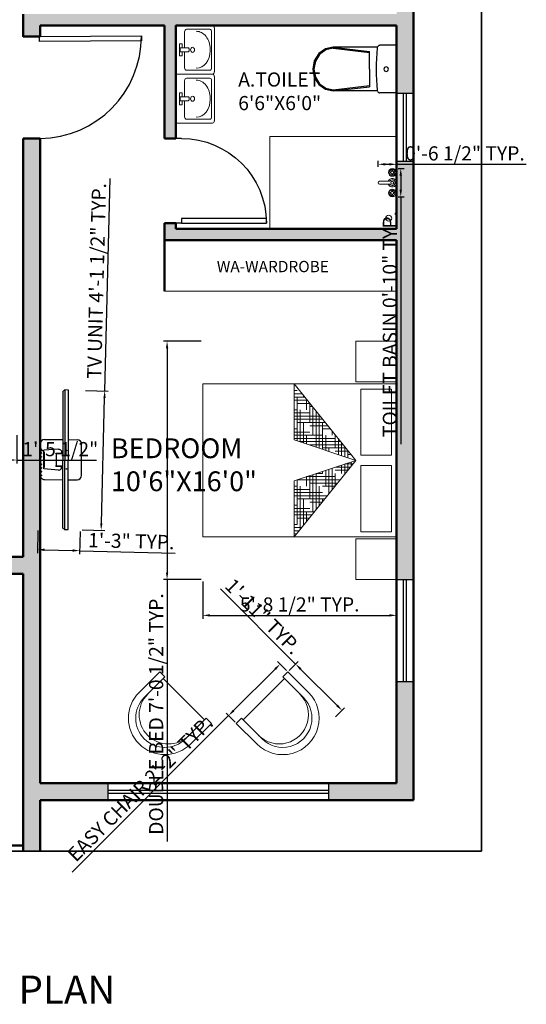
# Model space of a CAD drawing. Units: inches. Extents: x 2638 to 4577, y 1946 to 2619.
# Tile 5 of 8: x 3284 to 3463, y 1946 to 2294. Entities that reach past the tile are written whole.
import ezdxf

# ---------------------------------------------------------------- set-up
doc = ezdxf.new("R2010")
doc.units = ezdxf.units.IN
for name, color, linetype, lineweight in [('A-ANNO-DIMS', 2, 'Continuous', 18), ('A-ANNO-TEXT', 7, 'Continuous', 25), ('A-AREA-IDEN', 7, 'Continuous', 25), ('A-DOOR', 4, 'Continuous', 25), ('A-FLOR-FIXT', 8, 'Continuous', 18), ('A-FURN', 8, 'Continuous', 18), ('A-GLAZ', 4, 'Continuous', 25), ('A-WALL', 7, 'Continuous', 50), ('A-WALL-PATT', 8, 'Continuous', 13), ('C-PROP', 1, 'Continuous', 35)]:
    doc.layers.add(name, color=color, linetype=linetype, lineweight=lineweight)
doc.layers.add('SANTEH', color=7, linetype='Continuous')
doc.layers.add('window', color=130, linetype='Continuous')
doc.styles.get("Standard").update_dxf_attribs({"font": 'arial.ttf'})
doc.dimstyles.new('ISO-25', dxfattribs={"dimtxt": 5, "dimasz": 2.5, "dimexe": 1.25, "dimexo": 0.625, "dimtad": 1, "dimdec": 1, "dimlunit": 3, "dimtxsty": 'Standard', "dimcen": 2.5, "dimclrt": 1, "dimadec": 0, "dimazin": 0, "dimtfac": 1, "dimtdec": 1, "dimtmove": 0, "dimatfit": 3, "dimfxl": 1, "dimarcsym": 0})

# ---------------------------------------------------------------- blocks, each defined once
blk = doc.blocks.new('*U5')
for p, q in [((0, 0), (0, -6)), ((30, 0), (30, -6))]:
    blk.add_line(p, q)
blk.add_lwpolyline([(0, 0), (0, 30), (1.75, 30), (1.75, 0)], close=True)
blk.add_arc((0, 0), 30, 0, 90)
blk = doc.blocks.new('*U4')
for p, q in [((0, 0), (0, -6)), ((36, 0), (36, -6))]:
    blk.add_line(p, q)
blk.add_lwpolyline([(0, 0), (0, 36), (1.75, 36), (1.75, 0)], close=True)
blk.add_arc((0, 0), 36, 0, 90)
blk = doc.blocks.new('TV')
at = {"color": 0}
for p, q in [((3967.27, 1784.85), (3967.05, 1784.65)), ((3967.76, 1763.68), (3967.54, 1763.86))]:
    blk.add_line(p, q, dxfattribs=at)
at = {"layer": 'window'}
for p, q in [((3967.54, 1763.86), (3967.05, 1784.65)), ((3964.41, 1777.23), (3967.22, 1777.3)), ((3968.01, 1777.32), (3969.36, 1777.35)), ((3966.53, 1775.82), (3964.33, 1775.61)), ((3964.34, 1775.34), (3964.45, 1775.34)), ((3964.34, 1775.31), (3964.43, 1775.32)), ((3966.14, 1775.2), (3967.01, 1775.22)), ((3966.14, 1775.18), (3967.27, 1775.2)), ((3966.14, 1775.18), (3966.14, 1775.2)), ((3966.3, 1773.29), (3966.26, 1775.18)), ((3964.39, 1773.06), (3964.48, 1773.06)), ((3964.39, 1773.04), (3964.5, 1773.04)), ((3966.19, 1773.28), (3967.31, 1773.31)), ((3966.19, 1773.26), (3967.05, 1773.28)), ((3966.19, 1773.26), (3966.19, 1773.28)), ((3966.61, 1772.66), (3964.4, 1772.77)), ((3964.55, 1771.15), (3967.36, 1771.22)), ((3968.15, 1771.24), (3969.5, 1771.27))]:
    blk.add_line(p, q, dxfattribs=at)
for points in [[(3968.33, 1763.69), (3967.83, 1784.86), (3967.27, 1784.85), (3967.76, 1763.68), (3968.33, 1763.69)], [(3963.86, 1771.81), (3963.75, 1776.54)], [(3970.16, 1771.96), (3970.05, 1776.69)], [(3964.4, 1772.77), (3964.33, 1775.61)], [(3964.48, 1773.06), (3964.43, 1775.32)], [(3964.5, 1773.04), (3964.45, 1775.34)]]:
    blk.add_lwpolyline(points, dxfattribs=at)
for points in [[(3966.53, 1775.82, -0.263666), (3966.93, 1775.69), (3967, 1775.57), (3967.01, 1775.22)], [(3966.61, 1772.66, 0.263666), (3967, 1772.81), (3967.06, 1772.93), (3967.05, 1773.28)]]:
    blk.add_lwpolyline(points, format="xyb", dxfattribs=at)
for centre, radius in [((3963.91, 1775.73), 0.0679), ((3963.93, 1775.17), 0.0679), ((3963.94, 1774.6), 0.0679), ((3967.77, 1775.68), 0.0451), ((3963.95, 1774.04), 0.0679), ((3963.97, 1773.48), 0.0679), ((3963.98, 1772.92), 0.0679), ((3967.83, 1772.86), 0.0451), ((3963.99, 1772.35), 0.0679), ((3964.01, 1771.79), 0.0679)]:
    blk.add_circle(centre, radius, dxfattribs=at)
for centre, start, end in [((3964.42, 1776.56), 91.3414, 181.3414), ((3969.38, 1776.67), 1.3414, 91.3414), ((3964.53, 1771.83), 181.3414, 271.3414), ((3969.49, 1771.94), 271.3414, 1.3414)]:
    blk.add_arc(centre, 0.676, start, end, dxfattribs=at)
blk = doc.blocks.new('Rac7')
at = {"color": 0}
for p, q in [((-39501, -24232), (-39501, -23830)), ((-39474, -23808), (-38988, -23808)), ((-39457, -23859), (-39457, -24115)), ((-39032, -23838), (-39430, -23838)), ((-39221, -23855), (-39241, -23855)), ((-39005, -24115), (-39005, -23859)), ((-39005, -23859), (-39005, -23859)), ((-38961, -23830), (-38961, -24232)), ((-39253, -24186), (-39253, -24094)), ((-39209, -24186), (-39209, -24094)), ((-39430, -24136), (-39253, -24136)), ((-39297, -24164), (-39253, -24164)), ((-39297, -24194), (-39297, -24164)), ((-39165, -24194), (-39297, -24194)), ((-39253, -24186), (-39209, -24186)), ((-39209, -24136), (-39032, -24136)), ((-39209, -24164), (-39165, -24164)), ((-39165, -24164), (-39165, -24194)), ((-38961, -24232), (-39501, -24232))]:
    blk.add_line(p, q, dxfattribs=at)
at = {"color": 0, "extrusion": (0, 0, -1)}
for centre, major_axis, start_param, end_param in [((-39474, -23830), (-27, 0), 0, 1.570796), ((-39430, -23859), (-27, 0), 0, 1.570796), ((-39241, -24007), (-194, 0), 0, 1.570796), ((-39221, -24007), (-194, 0), 1.570796, 3.141593), ((-39032, -23859), (-27, 0), 1.570796, 3.141593), ((-38988, -23830), (-27, 0), 1.570796, 3.141593), ((-39231, -24104), (-25.3, 0), 0.552816, 2.588777), ((-39430, -24115), (-27, 0), -1.570796, 0), ((-39032, -24115), (-27, 0), -3.141593, -1.570796)]:
    blk.add_ellipse(centre, major_axis=major_axis, ratio=0.785714, start_param=start_param, end_param=end_param, dxfattribs=at)
blk.add_ellipse((-39231, -24048), major_axis=(-27.9, 0), ratio=0.785714, dxfattribs=at)
blk = doc.blocks.new('WC 2 Symb_109')
at = {"layer": 'SANTEH'}
for p, q in [((0, 0), (0, 380)), ((0, 380), (132.4, 380)), ((153.6, 364.9), (506.8, 364.9)), ((506.3, 364.9), (215.7, 330.9)), ((506.3, 356), (215.7, 322)), ((215.7, 190), (215.7, 330.9)), ((215.7, 190), (215.7, 49.1)), ((153.8, 15.1), (506.8, 15.1)), ((506.3, 24), (215.7, 58)), ((506.3, 15.1), (215.7, 49.1)), ((0, 0), (132.4, 0))]:
    blk.add_line(p, q, dxfattribs=at)
for points in [[(154.6, 360.1), (153.9, 364.1), (152.3, 367.9), (150.2, 371.3), (147.4, 374.3), (144.1, 376.7), (140.5, 378.5), (136.5, 379.6), (132.4, 380)], [(154.6, 19.7), (158.6, 62.1), (161.4, 104.7), (163.1, 147.3), (163.7, 189.9), (163.1, 232.5), (161.4, 275.1), (158.6, 317.7), (154.6, 360.1)], [(506.3, 24), (565.5, 36.6), (615.7, 72.6), (649.2, 126.5), (661, 190), (649.2, 253.5), (615.7, 307.4), (565.5, 343.4), (506.3, 356)], [(506.8, 15.1), (569.2, 28.4), (622.2, 66.3), (657.6, 123.1), (670, 190), (657.6, 256.9), (622.2, 313.7), (569.2, 351.6), (506.8, 364.9)], [(132.4, 0), (136.5, 0.4), (140.4, 1.5), (144.1, 3.2), (147.3, 5.6), (150.1, 8.6), (152.3, 12), (153.8, 15.7), (154.6, 19.7)]]:
    blk.add_lwpolyline(points, dxfattribs=at)
blk.add_lwpolyline([(83.6, 208.5), (70.4, 203.1), (64.9, 190), (70.4, 176.9), (83.6, 171.5), (96.8, 176.9), (102.2, 190), (96.8, 203.1)], close=True, dxfattribs=at)
blk = doc.blocks.new('Faucet - Bathroom top')
for p, q in [((-4.107, 0.125), (-4.375, 0.125)), ((-3.75, 0.4788), (-3.75, 0.75)), ((-3.5, 0.482), (-3.5, 0.75)), ((-3.1461, 0.125), (-2.875, 0.125)), ((3.143, 0.125), (2.875, 0.125)), ((3.5, 0.4788), (3.5, 0.75)), ((3.75, 0.482), (3.75, 0.75)), ((4.1039, 0.125), (4.375, 0.125)), ((-4.1039, -0.125), (-4.375, -0.125)), ((-3.75, -0.4821), (-3.75, -0.75)), ((-3.5, -0.4789), (-3.5, -0.75)), ((-3.143, -0.125), (-2.875, -0.125)), ((-0.5, -0.8639), (-0.5, -4.5)), ((0.5, -4.5), (0.5, -0.8631)), ((3.1461, -0.125), (2.875, -0.125)), ((3.5, -0.4821), (3.5, -0.75)), ((3.75, -0.4789), (3.75, -0.75)), ((4.107, -0.125), (4.375, -0.125))]:
    blk.add_line(p, q)
for centre, radius in [((-3.625, 0), 1.375), ((-4.625, 0), 0.2795), ((-3.625, 0), 0.5), ((-3.625, 1), 0.2795), ((-2.625, 0), 0.2795), ((0, 0), 0.5), ((3.625, 0), 1.375), ((2.625, 0), 0.2795), ((3.625, 0), 0.5), ((3.625, 1), 0.2795), ((4.625, 0), 0.2795), ((-3.625, -1), 0.2795), ((3.625, -1), 0.2795)]:
    blk.add_circle(centre, radius)
for centre, radius, start, end in [((-3.625, 0), 1, 105.2407, 164.2093), ((-3.625, 0), 1, 16.44125, 74.07887), ((0, 0), 1.5, 289.6514, 250.3603), ((0, 0), 1, 300.3431, 239.7554), ((3.625, 0), 1, 106.12, 164.0884), ((3.625, 0), 1, 16.23422, 73.90469), ((-3.625, 0), 1, 196.2342, 253.9047), ((-3.625, 0), 1, 286.12, 344.0884), ((3.625, 0), 1, 196.4413, 254.0789), ((3.625, 0), 1, 285.2407, 344.2093), ((0, -4.5), 0.5, 180, 0)]:
    blk.add_arc(centre, radius, start, end)
blk = doc.blocks.new('*X22')
at = {"color": 0}
for p, q in [((20.25, 14.8125), (20.2772, 14.8125)), ((20.1236, 14.6875), (20.25, 14.6875)), ((20.125, 14.5), (20.125, 14.6893)), ((20.1487, 14.7188), (20.2772, 14.7188)), ((20.1562, 14.625), (20.1562, 14.7281)), ((20.1739, 14.75), (20.2772, 14.75)), ((20.1875, 14.75), (20.1875, 14.7669)), ((20.199, 14.7812), (20.2772, 14.7812)), ((20.25, 14.3194), (20.25, 14.75)), ((20.0625, 14.2573), (20.0625, 14.6116)), ((20.0938, 14.375), (20.0938, 14.6504)), ((20.0984, 14.6562), (20.125, 14.6562)), ((20.125, 14.5938), (20.2772, 14.5938)), ((20.2188, 14.3091), (20.2188, 14.625)), ((20.25, 14.625), (20.2772, 14.625)), ((19.9727, 14.5), (20.25, 14.5)), ((19.9979, 14.5312), (20.2772, 14.5312)), ((20, 14.2366), (20, 14.5)), ((20.023, 14.5625), (20.2772, 14.5625)), ((20.0312, 14.2469), (20.0312, 14.5727)), ((20.1875, 14.2987), (20.1875, 14.5)), ((19.9062, 14.375), (19.9062, 14.4174)), ((19.9225, 14.4375), (20, 14.4375)), ((19.9476, 14.4688), (20.125, 14.4688)), ((20.125, 14.4062), (20.2772, 14.4062)), ((20.25, 14.4375), (20.2772, 14.4375)), ((19.8125, 14.1744), (19.8125, 14.3008)), ((19.8219, 14.3125), (20.2291, 14.3125)), ((19.8438, 14.1848), (19.8438, 14.3397)), ((19.875, 14.25), (19.875, 14.3785)), ((19.875, 14.3438), (20.2772, 14.3438)), ((19.9688, 14.2262), (19.9688, 14.375)), ((20, 14.375), (20.2772, 14.375)), ((20.1562, 14.2884), (20.1562, 14.375)), ((19.7465, 14.2188), (19.875, 14.2188)), ((19.75, 14.1537), (19.75, 14.2231)), ((19.7716, 14.25), (20, 14.25)), ((19.7812, 14.1641), (19.7812, 14.262)), ((19.7967, 14.2812), (20.125, 14.2812)), ((19.9375, 14.2159), (19.9375, 14.25)), ((19.7188, 14.0726), (19.7188, 14.1136)), ((19.7213, 14.1875), (19.75, 14.1875)), ((19.7018, 14.0938), (19.7786, 14.0938)), ((19.7269, 14.0625), (19.8728, 14.0625)), ((19.75, 14.0338), (19.75, 14.1032)), ((19.752, 14.0312), (19.875, 14.0312)), ((19.7812, 13.9949), (19.7812, 14.0929)), ((19.8125, 14), (19.8125, 14.0825)), ((19.9062, 13.8396), (19.9062, 14.0514)), ((19.9375, 13.8007), (19.9375, 14.0411)), ((19.9688, 13.875), (19.9688, 14.0307)), ((20, 14), (20, 14.0204)), ((19.8275, 13.9375), (20.25, 13.9375)), ((19.875, 13.8784), (19.875, 14)), ((19.875, 13.9688), (20.1557, 13.9688)), ((20, 14), (20.0614, 14)), ((20.0625, 13.6454), (20.0625, 13.9996)), ((20.0938, 13.625), (20.0938, 13.9893)), ((20.125, 13.75), (20.125, 13.9789)), ((20.1562, 13.875), (20.1562, 13.9686)), ((20.25, 13.5), (20.25, 13.9375)), ((19.8526, 13.9062), (20.125, 13.9062)), ((19.8777, 13.875), (20, 13.875)), ((20.0312, 13.6842), (20.0312, 13.875)), ((20.125, 13.8438), (20.2772, 13.8438)), ((20.2188, 13.4511), (20.2188, 13.875)), ((20.25, 13.875), (20.2772, 13.875)), ((19.9532, 13.7812), (20.2772, 13.7812)), ((19.9783, 13.75), (20.25, 13.75)), ((20, 13.8125), (20.2772, 13.8125)), ((20, 13.723), (20, 13.75)), ((20.1875, 13.49), (20.1875, 13.75)), ((20.0035, 13.7188), (20.125, 13.7188)), ((20.0789, 13.625), (20.2772, 13.625)), ((20.125, 13.6562), (20.2772, 13.6562)), ((20.1562, 13.5288), (20.1562, 13.625)), ((20.25, 13.6875), (20.2772, 13.6875)), ((20.104, 13.5938), (20.2772, 13.5938)), ((20.1292, 13.5625), (20.25, 13.5625)), ((20.2046, 13.4688), (20.2772, 13.4688)), ((20.2297, 13.4375), (20.2772, 13.4375)), ((20.25, 13.5), (20.2772, 13.5)), ((20.2549, 13.4062), (20.2772, 13.4062))]:
    blk.add_line(p, q, dxfattribs=at)
blk = doc.blocks.new('MAT-P02')
for p, q in [((-1.17, 0), (-1.17, -0.4)), ((-1.17, 0), (-0.77, 0)), ((-0.77, 0), (-0.77, -0.4)), ((-0.75, 0), (0.75, 0)), ((-0.75, 0), (-0.75, -1.9)), ((0.75, 0), (0.75, -1.9)), ((0.77, 0), (1.17, 0)), ((0.77, 0), (0.77, -0.4)), ((1.17, 0), (1.17, -0.4)), ((-0.7, -0.05), (-0.7, -0.35)), ((-0.7, -0.05), (-0.05, -0.05)), ((-0.05, -0.35), (-0.05, -0.05)), ((0.05, -0.05), (0.7, -0.05)), ((0.05, -0.35), (0.05, -0.05)), ((0.7, -0.05), (0.7, -0.35)), ((-0.7, -0.35), (-0.05, -0.35)), ((0.05, -0.35), (0.7, -0.35)), ((-1.17, -0.4), (-0.77, -0.4)), ((-0.75, -1.0034), (0, -0.4)), ((0, -0.4), (-0.75, -1.0034)), ((0, -0.4), (-0.2, -1.0034)), ((0, -0.4), (0.2, -1.0034)), ((0, -0.4), (0.75, -1.0034)), ((0.77, -0.4), (1.17, -0.4)), ((-0.75, -1.0034), (-0.2, -1.0034)), ((0.2, -1.0034), (0.75, -1.0034)), ((0.75, -1.9), (-0.75, -1.9))]:
    blk.add_line(p, q)
at = {"xscale": -1, "rotation": 90}
blk.add_blockref('*X22', (14.1285, 19.2738), dxfattribs=at)
blk = doc.blocks.new('12PSTG07')
at = {"color": 0, "linetype": 'ByBlock'}
for p, q in [((0, 15), (-12, 15)), ((0, 12), (0, 15)), ((-12, 12), (0, 12)), ((-1, -12), (-1, 12)), ((-12, -12), (0, -12)), ((0, -12), (0, -15)), ((0, -15), (-12, -15))]:
    blk.add_line(p, q, dxfattribs=at)
for centre, radius in [((-12, 0), 15), ((-12, 0), 12), ((-10, 0), 12)]:
    blk.add_arc(centre, radius, 90, 270, dxfattribs=at)
blk = doc.blocks.new('WIN-36')
for p, q in [((2761.41, 2540.16), (2761.41, 2534.16)), ((2797.41, 2540.16), (2797.41, 2534.16)), ((2761.41, 2537.66), (2797.41, 2537.66)), ((2761.41, 2536.66), (2797.41, 2536.66))]:
    blk.add_line(p, q)
blk = doc.blocks.new('WIN-24')
for p, q in [((2905.41, 2558.16), (2905.41, 2552.16)), ((2929.41, 2558.16), (2929.41, 2552.16)), ((2905.41, 2555.66), (2929.41, 2555.66)), ((2905.41, 2554.66), (2929.41, 2554.66))]:
    blk.add_line(p, q)
blk = doc.blocks.new('WIN-78')
for p, q in [((3314.99, 2024.16), (3314.99, 2018.16)), ((3392.99, 2024.16), (3392.99, 2018.16)), ((3314.99, 2021.66), (3392.99, 2021.66)), ((3314.99, 2020.66), (3392.99, 2020.66))]:
    blk.add_line(p, q)
blk = doc.blocks.new('*D59')
at = {"layer": 'A-ANNO-DIMS', "color": 0, "lineweight": -2, "transparency": 16777216}
for p, q in [((3378.15, 2064), (3374.97, 2067.18)), ((3374.09, 2064.53), (3359.39, 2049.82)), ((3357.62, 2048.05), (3302.31, 1992.75)), ((3359.91, 2045.76), (3356.74, 2048.94))]:
    blk.add_line(p, q, dxfattribs=at)
at = {"layer": 'A-ANNO-DIMS', "color": 0, "transparency": 16777216}
for points in [[(3373.8, 2064.82), (3374.39, 2064.23), (3375.86, 2066.29)], [(3359.09, 2050.12), (3359.68, 2049.53), (3357.62, 2048.05)]]:
    blk.add_solid(points, dxfattribs=at)
at = {"layer": 'Defpoints', "color": 0, "transparency": 16777216}
for p in [(3378.59, 2063.56), (3357.62, 2048.05), (3360.36, 2045.32)]:
    blk.add_point(p, dxfattribs=at)
at = {"layer": 'A-ANNO-DIMS', "color": 1, "transparency": 16777216, "insert": (3326.81, 2021.79), "char_height": 5, "attachment_point": 5, "rotation": 45}
blk.add_mtext('EASY CHAIR 2\'-2" TYP.', dxfattribs=at)
blk = doc.blocks.new('*D60')
at = {"layer": 'A-ANNO-DIMS', "color": 0, "lineweight": -2, "transparency": 16777216}
for p, q in [((3381.33, 2066.29), (3354.71, 2092.91)), ((3379.04, 2064), (3382.21, 2067.18)), ((3395.98, 2051.65), (3383.1, 2064.53)), ((3395.45, 2047.58), (3398.63, 2050.76))]:
    blk.add_line(p, q, dxfattribs=at)
at = {"layer": 'A-ANNO-DIMS', "color": 0, "transparency": 16777216}
for points in [[(3383.39, 2064.82), (3382.8, 2064.23), (3381.33, 2066.29)], [(3396.27, 2051.94), (3395.68, 2051.35), (3397.75, 2049.88)]]:
    blk.add_solid(points, dxfattribs=at)
at = {"layer": 'Defpoints', "color": 0, "transparency": 16777216}
for p in [(3381.33, 2066.29), (3378.59, 2063.56), (3395.01, 2047.14)]:
    blk.add_point(p, dxfattribs=at)
at = {"layer": 'A-ANNO-DIMS', "color": 1, "transparency": 16777216, "insert": (3369.36, 2082.7), "char_height": 5, "attachment_point": 5, "rotation": 315}
blk.add_mtext('1\'-11" TYP.', dxfattribs=at)
blk = doc.blocks.new('*D67')
at = {"layer": 'A-ANNO-DIMS', "color": 0, "lineweight": -2, "transparency": 16777216}
for p, q in [((3313.83, 2162.87), (3315.74, 2237.96)), ((3307.06, 2163.05), (3315.08, 2162.84)), ((3312.64, 2116.09), (3313.76, 2160.38)), ((3305.8, 2113.76), (3313.82, 2113.56))]:
    blk.add_line(p, q, dxfattribs=at)
at = {"layer": 'A-ANNO-DIMS', "color": 0, "transparency": 16777216}
for points in [[(3313.35, 2160.39), (3314.18, 2160.37), (3313.83, 2162.87)], [(3312.22, 2116.1), (3313.05, 2116.08), (3312.57, 2113.59)]]:
    blk.add_solid(points, dxfattribs=at)
at = {"layer": 'Defpoints', "color": 0, "transparency": 16777216}
for p in [(3306.43, 2163.06), (3313.83, 2162.87), (3305.18, 2113.78)]:
    blk.add_point(p, dxfattribs=at)
at = {"layer": 'A-ANNO-DIMS', "color": 1, "transparency": 16777216, "insert": (3311.6, 2201.75), "char_height": 5, "attachment_point": 5, "rotation": 88.5431}
blk.add_mtext('TV UNIT 4\'-1 1/2" TYP.', dxfattribs=at)
blk = doc.blocks.new('*D68')
at = {"layer": 'A-ANNO-DIMS', "color": 0, "lineweight": -2, "transparency": 16777216}
for p, q in [((3290.21, 2113.53), (3290.01, 2105.51)), ((3305.16, 2113.15), (3304.96, 2105.13)), ((3292.54, 2106.7), (3302.49, 2106.45)), ((3304.99, 2106.38), (3338.74, 2105.52))]:
    blk.add_line(p, q, dxfattribs=at)
at = {"layer": 'A-ANNO-DIMS', "color": 0, "transparency": 16777216}
for points in [[(3292.55, 2107.12), (3292.53, 2106.28), (3290.04, 2106.76)], [(3302.5, 2106.86), (3302.48, 2106.03), (3304.99, 2106.38)]]:
    blk.add_solid(points, dxfattribs=at)
at = {"layer": 'Defpoints', "color": 0, "transparency": 16777216}
for p in [(3290.23, 2114.16), (3305.18, 2113.78), (3304.99, 2106.38)]:
    blk.add_point(p, dxfattribs=at)
at = {"layer": 'A-ANNO-DIMS', "color": 1, "transparency": 16777216, "insert": (3323.2, 2109.1), "char_height": 5, "attachment_point": 5, "rotation": 358.5431}
blk.add_mtext('1\'-3" TYP.', dxfattribs=at)
blk = doc.blocks.new('*D71')
at = {"layer": 'A-ANNO-DIMS', "color": 0, "lineweight": -2, "transparency": 16777216}
for p, q in [((3417.62, 2241.52), (3419.74, 2241.52)), ((3418.49, 2239.02), (3418.49, 2234.02)), ((3417.62, 2231.52), (3419.74, 2231.52)), ((3418.49, 2231.52), (3418.49, 2143.99))]:
    blk.add_line(p, q, dxfattribs=at)
at = {"layer": 'A-ANNO-DIMS', "color": 0, "transparency": 16777216}
for points in [[(3418.07, 2239.02), (3418.91, 2239.02), (3418.49, 2241.52)], [(3418.07, 2234.02), (3418.91, 2234.02), (3418.49, 2231.52)]]:
    blk.add_solid(points, dxfattribs=at)
at = {"layer": 'Defpoints', "color": 0, "transparency": 16777216}
for p in [(3416.99, 2241.52), (3416.99, 2231.52), (3418.49, 2231.52)]:
    blk.add_point(p, dxfattribs=at)
at = {"layer": 'A-ANNO-DIMS', "color": 1, "transparency": 16777216, "insert": (3415.28, 2186.51), "char_height": 5, "attachment_point": 5, "rotation": 90}
blk.add_mtext('TOILET BASIN 0\'-10" TYP.', dxfattribs=at)
blk = doc.blocks.new('*D72')
at = {"layer": 'A-ANNO-DIMS', "color": 0, "lineweight": -2, "transparency": 16777216}
for p, q in [((3410.49, 2242.15), (3410.49, 2244.27)), ((3412.99, 2243.02), (3414.49, 2243.02)), ((3416.99, 2242.15), (3416.99, 2244.27)), ((3416.99, 2243.02), (3462.87, 2243.02))]:
    blk.add_line(p, q, dxfattribs=at)
at = {"layer": 'A-ANNO-DIMS', "color": 0, "transparency": 16777216}
for points in [[(3412.99, 2243.44), (3412.99, 2242.61), (3410.49, 2243.02)], [(3414.49, 2243.44), (3414.49, 2242.61), (3416.99, 2243.02)]]:
    blk.add_solid(points, dxfattribs=at)
at = {"layer": 'Defpoints', "color": 0, "transparency": 16777216}
for p in [(3416.99, 2243.02), (3410.49, 2241.52), (3416.99, 2241.52)]:
    blk.add_point(p, dxfattribs=at)
at = {"layer": 'A-ANNO-DIMS', "color": 1, "transparency": 16777216, "insert": (3441.18, 2246.23), "char_height": 5, "attachment_point": 5}
blk.add_mtext('0\'-6 1/2" TYP.', dxfattribs=at)
blk = doc.blocks.new('*D73')
at = {"layer": 'A-ANNO-DIMS', "color": 0, "lineweight": -2, "transparency": 16777216}
for p, q in [((3347.9, 2180.48), (3334.62, 2180.48)), ((3335.87, 2177.98), (3335.87, 2098.66)), ((3347.9, 2096.16), (3334.62, 2096.16)), ((3335.87, 2096.16), (3335.87, 2003.56))]:
    blk.add_line(p, q, dxfattribs=at)
at = {"layer": 'A-ANNO-DIMS', "color": 0, "transparency": 16777216}
for points in [[(3335.46, 2177.98), (3336.29, 2177.98), (3335.87, 2180.48)], [(3335.46, 2098.66), (3336.29, 2098.66), (3335.87, 2096.16)]]:
    blk.add_solid(points, dxfattribs=at)
at = {"layer": 'Defpoints', "color": 0, "transparency": 16777216}
for p in [(3348.52, 2180.48), (3335.87, 2096.16), (3348.52, 2096.16)]:
    blk.add_point(p, dxfattribs=at)
at = {"layer": 'A-ANNO-DIMS', "color": 1, "transparency": 16777216, "insert": (3332.66, 2048.61), "char_height": 5, "attachment_point": 5, "rotation": 90}
blk.add_mtext('DOUBLE BED 7\'-0 1/2" TYP.', dxfattribs=at)
blk = doc.blocks.new('*D74')
at = {"layer": 'A-ANNO-DIMS', "color": 0, "lineweight": -2, "transparency": 16777216}
for p, q in [((3348.52, 2095.53), (3348.52, 2082.26)), ((3416.99, 2095.53), (3416.99, 2082.26)), ((3351.02, 2083.51), (3414.49, 2083.51))]:
    blk.add_line(p, q, dxfattribs=at)
at = {"layer": 'A-ANNO-DIMS', "color": 0, "transparency": 16777216}
for points in [[(3351.02, 2083.92), (3351.02, 2083.09), (3348.52, 2083.51)], [(3414.49, 2083.92), (3414.49, 2083.09), (3416.99, 2083.51)]]:
    blk.add_solid(points, dxfattribs=at)
at = {"layer": 'Defpoints', "color": 0, "transparency": 16777216}
for p in [(3348.52, 2096.16), (3416.99, 2096.16), (3416.99, 2083.51)]:
    blk.add_point(p, dxfattribs=at)
at = {"layer": 'A-ANNO-DIMS', "color": 1, "transparency": 16777216, "insert": (3382.76, 2086.72), "char_height": 5, "attachment_point": 5}
blk.add_mtext('5\'-8 1/2" TYP.', dxfattribs=at)
blk = doc.blocks.new('*D76')
at = {"layer": 'A-ANNO-DIMS', "color": 0, "lineweight": -2, "transparency": 16777216}
for p, q in [((3265.04, 2147.27), (3265.04, 2137.19)), ((3282.76, 2147.27), (3282.76, 2137.19)), ((3267.54, 2138.44), (3280.26, 2138.44)), ((3282.76, 2138.44), (3310.98, 2138.44))]:
    blk.add_line(p, q, dxfattribs=at)
at = {"layer": 'A-ANNO-DIMS', "color": 0, "transparency": 16777216}
for points in [[(3267.54, 2138.86), (3267.54, 2138.03), (3265.04, 2138.44)], [(3280.26, 2138.86), (3280.26, 2138.03), (3282.76, 2138.44)]]:
    blk.add_solid(points, dxfattribs=at)
at = {"layer": 'Defpoints', "color": 0, "transparency": 16777216}
for p in [(3265.04, 2147.89), (3282.76, 2147.89), (3282.76, 2138.44)]:
    blk.add_point(p, dxfattribs=at)
at = {"layer": 'A-ANNO-DIMS', "color": 1, "transparency": 16777216, "insert": (3298.12, 2141.65), "char_height": 5, "attachment_point": 5}
blk.add_mtext('1\'-5 1/2"', dxfattribs=at)

msp = doc.modelspace()

# ---------------------------------------------------------------- hatches: boundary and pattern name
at = {"layer": 'A-WALL-PATT', "transparency": 33554687}
h = msp.add_hatch(color=256, dxfattribs=at)
h.dxf.hatch_style = 1
h.paths.add_polyline_path([(3116.99, 2552.16), (3137.99, 2552.16), (3137.99, 2558.16), (3110.99, 2558.16), (3110.99, 2507.16), (3116.99, 2507.16)])
h.paths.add_polyline_path([(3252.94, 2558.16), (3179.99, 2558.16), (3179.99, 2552.16), (3194.4, 2552.16), (3252.94, 2552.16)])
h.paths.add_polyline_path([(3422.99, 2558.16), (3288.94, 2558.16), (3288.94, 2552.16), (3318.99, 2552.16), (3318.99, 2532.16), (3322.99, 2532.16), (3322.99, 2552.16), (3416.99, 2552.16), (3416.99, 2492.16), (3354.99, 2492.16), (3354.99, 2488.16), (3416.99, 2488.16), (3416.99, 2481.16), (3422.99, 2481.16)])
h.paths.add_polyline_path([(3422.99, 2457.16), (3416.99, 2457.16), (3416.99, 2426.16), (3372.26, 2426.16), (3322.99, 2426.16), (3322.99, 2439.06), (3322.99, 2488.16), (3324.99, 2488.16), (3324.99, 2492.16), (3322.99, 2492.16), (3322.99, 2502.16), (3318.99, 2502.16), (3318.99, 2426.16), (3297.01, 2426.16), (3296.99, 2422.16), (3416.99, 2422.16), (3416.99, 2418.91), (3422.99, 2418.91)])
h.paths.add_polyline_path([(3146.99, 2104.16), (3116.99, 2104.16), (3116.99, 2116.16), (3110.99, 2116.16), (3110.99, 2098.16), (3146.99, 2098.16)])
h.paths.add_polyline_path([(3236.99, 2104.16), (3224.99, 2104.16), (3224.99, 2098.16), (3236.99, 2098.16)])
h.paths.add_polyline_path([(3290.99, 2252.16), (3284.99, 2252.16), (3284.99, 2104.16), (3278.99, 2104.16), (3278.99, 2098.16), (3284.99, 2098.16), (3284.99, 2000.16), (3290.99, 2000.16), (3290.99, 2018.16), (3314.99, 2018.16), (3314.99, 2024.16), (3290.99, 2024.16)])
h.paths.add_polyline_path([(3422.99, 2060.16), (3416.99, 2060.16), (3416.99, 2024.16), (3392.99, 2024.16), (3392.99, 2018.16), (3422.99, 2018.16)])
h.paths.add_polyline_path([(3422.99, 2244.16), (3416.99, 2244.16), (3416.99, 2220.16), (3372.26, 2220.16), (3338.99, 2220.16), (3338.99, 2222.16), (3334.99, 2222.16), (3334.99, 2216.16), (3416.99, 2216.16), (3416.99, 2096.16), (3422.99, 2096.16)])
h.paths.add_polyline_path([(3422.99, 2300.41), (3416.99, 2300.41), (3416.99, 2296.16), (3284.99, 2296.16), (3284.99, 2288.16), (3290.99, 2288.16), (3290.99, 2292.16), (3334.99, 2292.16), (3334.99, 2252.16), (3338.99, 2252.16), (3338.99, 2292.16), (3416.99, 2292.16), (3416.99, 2268.16), (3422.99, 2268.16)])
h.paths.add_polyline_path([(3422.99, 2382.91), (3416.99, 2382.91), (3416.99, 2336.41), (3422.99, 2336.41)])
h.paths.add_polyline_path([(3260.99, 2426.16), (3116.99, 2426.16), (3116.99, 2471.16), (3110.99, 2471.16), (3110.99, 2404.16), (3116.99, 2404.16), (3116.99, 2422.16), (3260.99, 2422.16)])
h.paths.add_polyline_path([(3116.99, 2320.16), (3110.99, 2320.16), (3110.99, 2152.16), (3116.99, 2152.16)])
h.paths.add_polyline_path([(3192.92, 2481.2), (3252.23, 2481.2), (3252.23, 2507.82), (3192.92, 2507.82)], flags=9)
h.paths.add_polyline_path([(3352.38, 2202.6), (3398.15, 2202.6), (3398.15, 2210.84), (3352.38, 2210.84)], flags=25)
h.paths.add_polyline_path([(3108.13, 2334.43), (3108.13, 2401.53), (3093.19, 2401.53), (3093.19, 2334.43)], flags=9)
h.paths.add_polyline_path([(3441.94, 2334.43), (3441.94, 2401.53), (3426.99, 2401.53), (3426.99, 2334.43)], flags=9)
h.paths.add_polyline_path([(3282.12, 2570.46), (3349.22, 2570.46), (3349.22, 2585.4), (3282.12, 2585.4)], flags=9)
h.paths.add_polyline_path([(3240.15, 2347.41), (3289.11, 2347.41), (3289.11, 2374.03), (3240.15, 2374.03)], flags=9)
h.paths.add_polyline_path([(3169.91, 2226.85), (3224.05, 2226.85), (3224.05, 2253.46), (3169.91, 2253.46)], flags=9)
h.paths.add_polyline_path([(3209.4, 2038.68), (3263.9, 2038.68), (3263.9, 2065.29), (3209.4, 2065.29)], flags=9)
h.paths.add_polyline_path([(3313.05, 2123.44), (3369.27, 2123.44), (3369.27, 2150.05), (3313.05, 2150.05)], flags=9)
h.paths.add_polyline_path([(3359.46, 2259.32), (3395.23, 2259.32), (3395.23, 2278.33), (3359.46, 2278.33)], flags=25)

# ---------------------------------------------------------------- linework, layer by layer
at = {"layer": 'A-FLOR-FIXT', "ltscale": 5}
msp.add_line((3372.26, 2252.89), (3372.26, 2220.16), dxfattribs=at)
msp.add_lwpolyline([(3372.26, 2220.16), (3416.99, 2220.16), (3416.99, 2252.89), (3372.26, 2252.89)], close=True, dxfattribs=at)
msp.add_circle((3414.24, 2223.96), 1.06, dxfattribs=at)
at = {"layer": 'A-FURN'}
msp.add_line((3416.99, 2198.16), (3334.99, 2198.16), dxfattribs=at)
at = {"layer": 'A-WALL'}
for p, q in [((3422.99, 2558.16), (3422.99, 2018.16)), ((3284.99, 2296.16), (3284.99, 2288.16)), ((3290.99, 2292.16), (3290.99, 2288.16)), ((3334.99, 2292.16), (3290.99, 2292.16)), ((3334.99, 2292.16), (3334.99, 2252.16)), ((3416.99, 2292.16), (3338.99, 2292.16)), ((3338.99, 2292.16), (3338.99, 2252.16)), ((3416.99, 2292.16), (3416.99, 2220.16)), ((3290.99, 2288.16), (3284.99, 2288.16)), ((3284.99, 2252.16), (3284.99, 2104.16)), ((3290.99, 2252.16), (3284.99, 2252.16)), ((3290.99, 2252.16), (3290.99, 2024.16)), ((3338.99, 2252.16), (3334.99, 2252.16)), ((3334.99, 2222.16), (3334.99, 2198.16)), ((3338.99, 2222.16), (3334.99, 2222.16)), ((3338.99, 2222.16), (3338.99, 2220.16)), ((3416.99, 2220.16), (3338.99, 2220.16)), ((3416.99, 2216.16), (3334.99, 2216.16)), ((3416.99, 2216.16), (3416.99, 2024.16)), ((3284.99, 2104.16), (3116.99, 2104.16)), ((3284.99, 2098.16), (3110.99, 2098.16)), ((3284.99, 2098.16), (3284.99, 2000.16)), ((3416.99, 2024.16), (3290.99, 2024.16)), ((3422.99, 2018.16), (3290.99, 2018.16)), ((3290.99, 2018.16), (3290.99, 2000.16)), ((3284.99, 2002.16), (3112.99, 2002.16))]:
    msp.add_line(p, q, dxfattribs=at)
at = {"layer": 'C-PROP'}
msp.add_lwpolyline([(3086.99, 2600.16), (3446.99, 2600.16), (3446.99, 2000.16), (3086.99, 2000.16)], close=True, dxfattribs=at)

# ---------------------------------------------------------------- block references
at = {"layer": 'A-DOOR', "rotation": 270.3213350750104}
msp.add_blockref('*U4', (3290.79, 2288.19), dxfattribs=at)
at = {"layer": 'A-DOOR', "xscale": -1, "rotation": 270}
msp.add_blockref('*U5', (3340.99, 2222.16), dxfattribs=at)
at = {"layer": 'A-FLOR-FIXT'}
for name, p, xscale, yscale, zscale, rotation in [('Rac7', (4116.04, 3541.53), -0.0320670790485951, 0.0320670790485951, 0.0320670790485951, 270), ('WC 2 Symb_109', (3416.99, 2285.09), 0.0441898926459964, 0.0441898926459964, 0.0441898926459964, 180), ('Rac7', (4116.04, 3524.24), -0.0320670790485951, 0.0320670790485951, 0.0320670790485951, 270)]:
    msp.add_blockref(name, p, dxfattribs=dict(at, xscale=xscale, yscale=yscale, zscale=zscale, rotation=rotation))
at = {"layer": 'A-FLOR-FIXT', "rotation": 270}
msp.add_blockref('Faucet - Bathroom top', (3415.49, 2236.52), dxfattribs=at)
at = {"layer": 'A-FURN'}
for name, p, xscale, yscale, zscale, rotation in [('MAT-P02', (3416.99, 2138.32), 36.03633950593442, 36.03633950593442, 36.03633950593442, 270), ('TV', (-6036.04, -1754.61), 2.327319231123021, 2.327319231123021, 2.327319231123021, 358.5430845181613), ('12PSTG07', (3342.41, 2054.44), -0.8597921787217943, 0.8597921787217943, 0.8597921787217943, 225), ('12PSTG07', (3369.47, 2054.44), 0.8597921787217943, 0.8597921787217943, 0.8597921787217943, 134.9999999999999)]:
    msp.add_blockref(name, p, dxfattribs=dict(at, xscale=xscale, yscale=yscale, zscale=zscale, rotation=rotation))
at = {"layer": 'A-GLAZ'}
for name, p, rotation in [('WIN-24', (5975.15, -661.25), 90.00000000000873), ('WIN-36', (5957.15, -701.25), 90.00000000000281)]:
    msp.add_blockref(name, p, dxfattribs=dict(at, rotation=rotation))
msp.add_blockref('WIN-78', (0, 0), dxfattribs=at)

# ---------------------------------------------------------------- texts
at = {"layer": 'A-ANNO-TEXT', "attachment_point": 1}
for s, width, insert, char_height in [('WA-WARDROBE', 29.5334, (3353.45, 2208.86), 4), ('{\\fTimes New Roman|b0|i0|c0|p18;FIRST FLOOR PLAN}', 196.2607, (3196.91, 1956.14), 10)]:
    msp.add_mtext_dynamic_manual_height_columns(s, width=width, gutter_width=12.5, heights=[0], dxfattribs=dict(at, insert=insert, char_height=char_height))
at = {"layer": 'A-AREA-IDEN', "attachment_point": 1}
for s, insert, char_height in [('{\\fTimes New Roman|b0|i0|c0|p18;A.TOILET\\P6\'6"X6\'0"}', (3361.03, 2275.5), 5), ('{\\fTimes New Roman|b0|i0|c0|p18;BEDROOM\\P10\'6"X16\'0"}', (3316.01, 2146.09), 7)]:
    msp.add_mtext_dynamic_manual_height_columns(s, width=61.0557, gutter_width=12.5, heights=[0], dxfattribs=dict(at, insert=insert, char_height=char_height))

# ---------------------------------------------------------------- dimensions: what is measured, and where the dimension line sits
at = {"layer": 'A-ANNO-DIMS'}
for base, p1, p2, picture, middle in [((3416.99, 2243.02), (3410.49, 2241.52), (3416.99, 2241.52), '*D72', (3441.18, 2246.23)), ((3416.99, 2083.51), (3348.52, 2096.16), (3416.99, 2096.16), '*D74', (3382.76, 2086.72))]:
    dim = msp.add_linear_dim(base=base, p1=p1, p2=p2, text='<> TYP.', dimstyle='ISO-25', override={"dimdec": 1, "dimrnd": 0, "dimzin": 1, "dimlunit": 4, "dimfrac": 2}, dxfattribs=at)
    dim.commit()
    dim.dimension.update_dxf_attribs({"geometry": picture, "text_midpoint": middle})
for base, p1, p2, angle, text, picture, middle in [((3418.49, 2231.52), (3416.99, 2241.52), (3416.99, 2231.52), 270, 'TOILET BASIN <> TYP.', '*D71', (3415.28, 2186.51)), ((3313.83, 2162.87), (3305.18, 2113.78), (3306.43, 2163.06), 88.5431, 'TV UNIT <> TYP.', '*D67', (3311.6, 2201.75)), ((3335.87, 2096.16), (3348.52, 2180.48), (3348.52, 2096.16), 270, 'DOUBLE BED <> TYP.', '*D73', (3332.66, 2048.61)), ((3304.99, 2106.38), (3290.23, 2114.16), (3305.18, 2113.78), 358.5431, '<> TYP.', '*D68', (3323.2, 2109.1)), ((3381.33, 2066.29), (3395.01, 2047.14), (3378.59, 2063.56), 135, '<> TYP.', '*D60', (3369.36, 2082.7)), ((3357.62, 2048.05), (3378.59, 2063.56), (3360.36, 2045.32), 225, 'EASY CHAIR <> TYP.', '*D59', (3326.81, 2021.79))]:
    dim = msp.add_linear_dim(base=base, p1=p1, p2=p2, angle=angle, text=text, dimstyle='ISO-25', override={"dimdec": 1, "dimrnd": 0, "dimzin": 1, "dimlunit": 4, "dimfrac": 2}, dxfattribs=at)
    dim.commit()
    dim.dimension.update_dxf_attribs({"geometry": picture, "text_midpoint": middle})
dim = msp.add_linear_dim(base=(3282.76, 2138.44), p1=(3265.04, 2147.89), p2=(3282.76, 2147.89), dimstyle='ISO-25', override={"dimdec": 1, "dimrnd": 0, "dimzin": 1, "dimlunit": 4, "dimfrac": 2}, dxfattribs=at)
dim.commit()
dim.dimension.update_dxf_attribs({"geometry": '*D76', "text_midpoint": (3298.12, 2141.65)})

doc.saveas('drawing.dxf')
